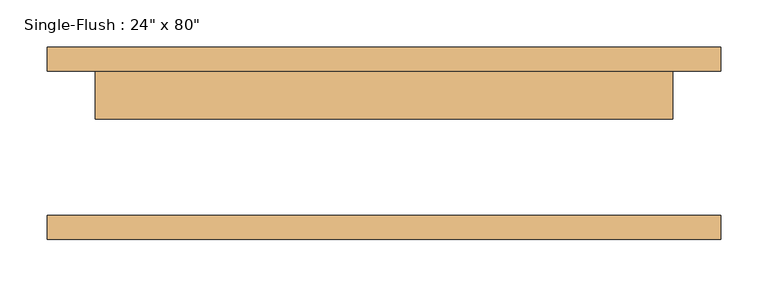
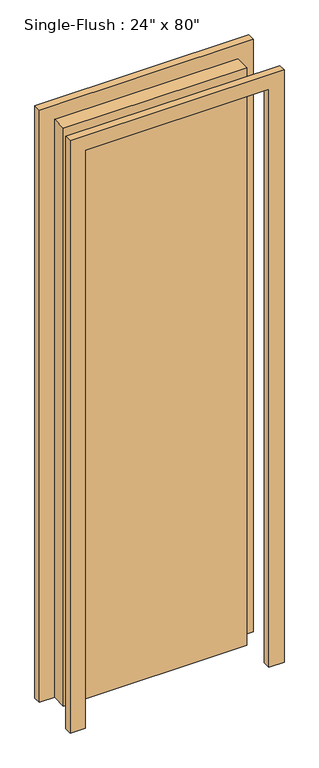
"""IFC4 building model written with IfcOpenShell, lengths in millimetres: door geometry."""

from ifc_helpers import new_model, si_unit, frame, origin, origin_with_axes, place, context, project, spatial, polyline, outline, extrude, source, transform, mapped, element, save


def door_d7591924(model_context):
    return source(origin(), model_context, "Body", "SweptSolid", [
        extrude(outline(polyline([(2082.8, -355.6), (0.0, -355.6), (0.0, -304.8), (2032.0, -304.8), (2032.0, 304.8), (0.0, 304.8), (0.0, 355.6), (2082.8, 355.6), (2082.8, -355.6)])), frame((0.0, 76.2, 0.0), z_axis=(0.0, 1.0, 0.0), x_axis=(0.0, 0.0, 1.0)), (0.0, 0.0, 1.0), 25.4),
        extrude(outline(polyline([(2082.8, 355.6), (2082.8, -355.6), (0.0, -355.6), (0.0, -304.8), (2032.0, -304.8), (2032.0, 304.8), (0.0, 304.8), (0.0, 355.6), (2082.8, 355.6)])), frame((0.0, -101.6, 0.0), z_axis=(0.0, 1.0, 0.0), x_axis=(0.0, 0.0, 1.0)), (0.0, 0.0, 1.0), 25.4),
        extrude(outline(polyline([(304.8, 25.4), (-304.8, 25.4), (-304.8, 76.2), (304.8, 76.2), (304.8, 25.4)])), origin_with_axes(), (0.0, 0.0, 1.0), 2032.0),
    ])


if __name__ == "__main__":
    model = new_model("IFC4")
    model_context = context("Model", 3, world=origin())
    ifc_project = project(units=[si_unit("LENGTHUNIT", "METRE", prefix="MILLI")], contexts=[model_context])
    site = spatial("IfcSite", under=ifc_project)
    building = spatial("IfcBuilding", under=site)
    placement = place(None, origin())
    door_shape = door_d7591924(model_context)
    element("IfcDoor", 1, ObjectType="Single-Flush : 24\" x 80\"", at=placement, inside=building, context=model_context, shape_type="MappedRepresentation", body=[
        mapped(door_shape, transform((0.0, 0.0, 0.0), x_axis=(1.0, 0.0, 0.0), y_axis=(0.0, 1.0, 0.0), z_axis=(0.0, 0.0, 1.0))),
    ])
    save(model, "model.ifc")

# Revit data of these elements
# Type "Single-Flush : 24\" x 80\""
#   Type Mark = "9"
#   Construction Type Id = "MDOOR"
#   Assembly Code = "C1020"
#   Analytic Construction = "Metal"
#   Thickness = 0' - 2"
#   Heat Transfer Coefficient (U) = 0.651978 BTU/(h·ft²·°F)
#   Height = 6' - 8"
#   Trim Projection Ext = 0' - 1"
#   Trim Projection Int = 0' - 1"
#   Trim Width = 0' - 2"
#   Width = 2' - 0"
#   Define Thermal Properties by = 1
#   Door Material = Door - Panel
#   Frame Material = Door - Frame
#   Visual Light Transmittance = 0
#   Solar Heat Gain Coefficient = 0
#   Function = (empty or 0)
#   Wall Closure = (empty or 0)
# Element 1 (IfcDoor, "Single-Flush : 24\" x 80\"")
#   Materials on its faces: "Door - Frame", "Door - Panel"
# Materials
#   "Door - Panel": class "Wood", colour RGB 210 159 95, transparency 0
#   "Door - Frame": colour RGB 118 70 51, transparency 0
